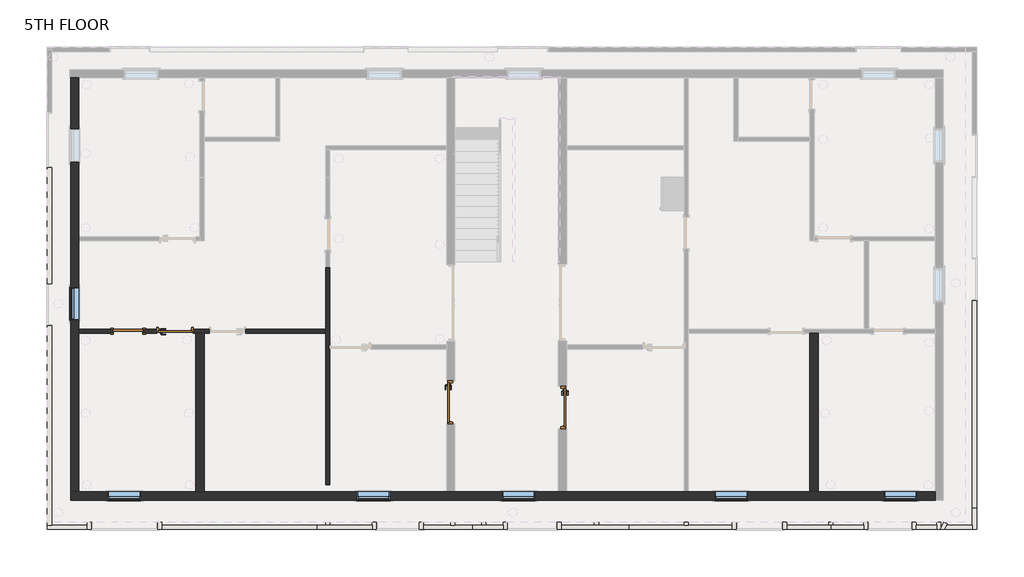
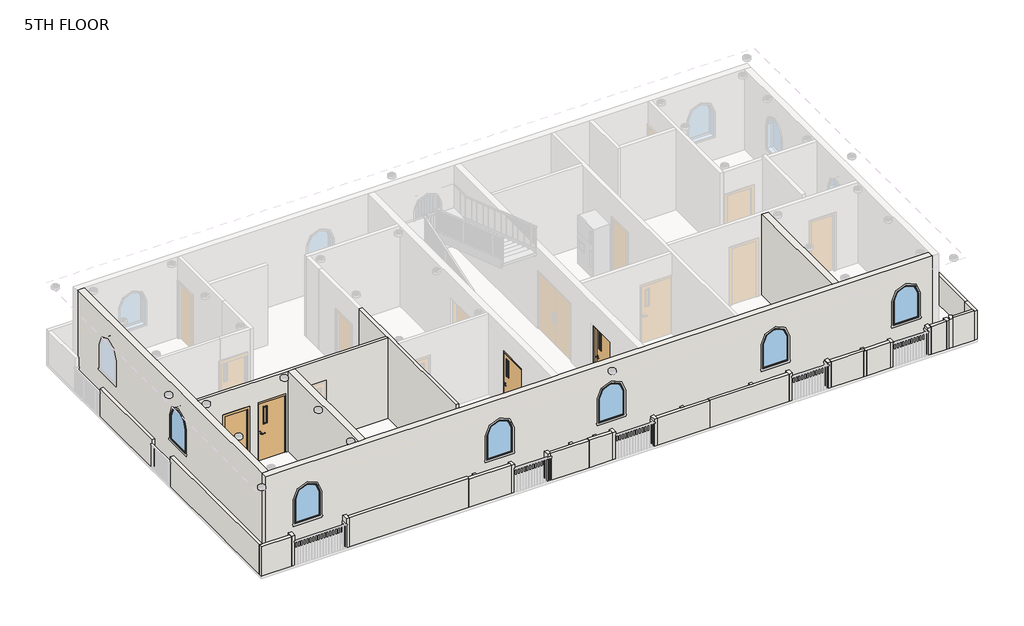
# One storey, part 1 of 7: 39 walls, 6 windows, 4 doors.
"""IFC4 building model written with IfcOpenShell, lengths in millimetres."""

from ifc_helpers import new_model, si_unit, frame, origin, place, context, project, spatial, polyline, circle_curve, outline, extrude, faceted_brep, transform, mapped, element, save
from ifc_brep_helpers import plane_surface, revolved_surface, advanced_brep
from components import door_586e558e, door_7d8f8091, door_passage_single_vision_lite_3_x7_38248cdf, door_d141acb4, window_fixed_round_top_3_x_4_dee2be1c

model = new_model("IFC4")

# Units and contexts
model_context = context("Model", 3, world=origin())
ifc_project = project(units=[si_unit("LENGTHUNIT", "METRE", prefix="MILLI")], contexts=[model_context])

# Site, building, storey
site = spatial("IfcSite", under=ifc_project)
building = spatial("IfcBuilding", under=site)
storey = spatial("IfcBuildingStorey", under=building, Name="5TH FLOOR", Elevation=16002.0)

# Doors
placement = place(None, origin())
door_shape = door_586e558e(model_context)
element("IfcDoor", 1, ObjectType="Door-Passage-Single-Vision_Lite : 3'6\"X7' 2", at=placement, inside=storey, context=model_context, shape_type="MappedRepresentation", body=[
    mapped(door_shape, transform((1116.1432011, -1461.3932193, 16002.0), x_axis=(0.0, -1.0, 0.0), y_axis=(1.0, 0.0, 0.0), z_axis=(0.0, 0.0, 1.0))),
])
door_2_shape = door_7d8f8091(model_context)
element("IfcDoor", 2, ObjectType="Door-Passage-Single-Vision_Lite : 3'7\"X7' 3", at=placement, inside=storey, context=model_context, shape_type="MappedRepresentation", body=[
    mapped(door_2_shape, transform((-1956.7487998, -1318.7421379, 16002.0), x_axis=(0.0, -1.0, 0.0), y_axis=(1.0, 0.0, 0.0), z_axis=(0.0, 0.0, 1.0))),
])
door_passage_single_vision_lite_3_x7_shape = door_passage_single_vision_lite_3_x7_38248cdf(model_context)
element("IfcDoor", 3, ObjectType="Door-Passage-Single-Vision_Lite : 3'X7'", at=placement, inside=storey, context=model_context, shape_type="MappedRepresentation", body=[
    mapped(door_passage_single_vision_lite_3_x7_shape, transform((-9570.3987992, 646.8067334, 16002.0), x_axis=(1.0, 0.0, 0.0), y_axis=(0.0, 1.0, 0.0), z_axis=(0.0, 0.0, 1.0))),
])
door_3_shape = door_d141acb4(model_context)
element("IfcDoor", 4, ObjectType="Single-Flush : 2'8\"x 7'", at=placement, inside=storey, context=model_context, shape_type="MappedRepresentation", body=[
    mapped(door_3_shape, transform((-10865.7987992, 640.4567334, 16002.0), x_axis=(1.0, 0.0, 0.0), y_axis=(0.0, 1.0, 0.0), z_axis=(0.0, 0.0, 1.0))),
])

# Walls
element("IfcWall", 5, ObjectType="Generic - 4.5\"", at=placement, inside=storey, context=model_context, shape_type="Brep", body=[
    faceted_brep([(-10459.3987992, 583.3067334, 18135.6), (-10459.3987992, 583.3067334, 16002.0), (-10078.3987992, 583.3067334, 16002.0), (-10078.3987992, 583.3067334, 18237.2), (-9062.3987992, 583.3067334, 18237.2), (-9062.3987992, 583.3067334, 16002.0), (-8998.8987992, 583.3067334, 16002.0), (-8770.2987992, 583.3067334, 16002.0), (-8630.5987992, 583.3067334, 16002.0), (-8630.5987992, 583.3067334, 18237.2), (-7614.5987992, 583.3067334, 18237.2), (-7614.5987992, 583.3067334, 16002.0), (-5417.4987995, 583.3067334, 16002.0), (-5417.4987995, 583.3067334, 19050.0), (-8770.2987992, 583.3067334, 19050.0), (-8998.8987992, 583.3067334, 19050.0), (-12224.6987925, 583.3067334, 19050.0), (-12224.6987925, 583.3067334, 16002.0), (-11272.1987992, 583.3067334, 16002.0), (-11272.1987992, 583.3067334, 18135.6), (-10078.3987992, 697.6067334, 16002.0), (-10459.3987992, 697.6067334, 16002.0), (-10459.3987992, 697.6067334, 18135.6), (-11272.1987992, 697.6067334, 18135.6), (-11272.1987992, 697.6067334, 16002.0), (-12224.6987925, 697.6067334, 16002.0), (-12224.6987925, 697.6067334, 19050.0), (-5417.4987995, 697.6067334, 19050.0), (-5417.4987995, 697.6067334, 16002.0), (-7614.5987992, 697.6067334, 16002.0), (-7614.5987992, 697.6067334, 18237.2), (-8630.5987992, 697.6067334, 18237.2), (-8630.5987992, 697.6067334, 16002.0), (-9062.3987992, 697.6067334, 16002.0), (-9062.3987992, 697.6067334, 18237.2), (-10078.3987992, 697.6067334, 18237.2)], [[[0, 1, 2, 3, 4, 5, 6, 7, 8, 9, 10, 11, 12, 13, 14, 15, 16, 17, 18, 19]], [[20, 21, 22, 23, 24, 25, 26, 27, 28, 29, 30, 31, 32, 33, 34, 35]], [[28, 12, 11, 29]], [[32, 8, 7, 6, 5, 33]], [[18, 17, 25, 24]], [[2, 1, 21, 20]], [[16, 15, 14, 13, 27, 26]], [[17, 16, 26, 25]], [[13, 12, 28, 27]], [[9, 8, 32, 31]], [[10, 9, 31, 30]], [[11, 10, 30, 29]], [[4, 34, 33, 5]], [[34, 4, 3, 35]], [[35, 3, 2, 20]], [[22, 21, 1, 0]], [[23, 22, 0, 19]], [[24, 23, 19, 18]]]),
])
element("IfcWall", 6, ObjectType="Generic - 4.5\"", at=placement, inside=storey, context=model_context, shape_type="Brep", body=[
    faceted_brep([(-5417.4987995, 2399.4067802, 16002.0), (-5417.4987995, 697.6067334, 16002.0), (-5417.4987995, 583.3067334, 16002.0), (-5417.4987995, -3594.9932193, 16002.0), (-5417.4987995, -3594.9932193, 19050.0), (-5417.4987995, 583.3067334, 19050.0), (-5417.4987995, 697.6067334, 19050.0), (-5417.4987995, 2399.4067802, 19050.0), (-5303.1987995, -3594.9932193, 19050.0), (-5303.1987995, -3594.9932193, 16002.0), (-5303.1987995, 148.1078621, 16002.0), (-5303.1987995, 148.1078621, 18237.2), (-5303.1987995, 262.4078621, 18237.2), (-5303.1987995, 262.4078621, 16002.0), (-5303.1987995, 2399.4067802, 16002.0), (-5303.1987995, 2399.4067802, 19050.0), (-5303.1987995, 262.4078621, 19050.0), (-5303.1987995, 148.1078621, 19050.0), (-5334.9487995, 262.4078621, 16002.0), (-5334.9487995, 148.1078621, 16002.0), (-5334.9487995, 262.4078621, 18237.2), (-5334.9487995, 148.1078621, 18237.2)], [[[0, 1, 2, 3, 4, 5, 6, 7]], [[8, 9, 10, 11, 12, 13, 14, 15, 16, 17]], [[3, 2, 1, 0, 14, 13, 18, 19, 10, 9]], [[4, 3, 9, 8]], [[7, 6, 5, 4, 8, 17, 16, 15]], [[0, 7, 15, 14]], [[20, 18, 13, 12]], [[19, 21, 11, 10]], [[21, 20, 12, 11]], [[18, 20, 21, 19]]]),
])
element("IfcWall", 7, ObjectType="Generic - 4.5\"", at=placement, inside=storey, context=model_context, shape_type="Brep", body=[
    faceted_brep([(-13088.8067989, -4826.8932661, 16002.0), (-11996.6067989, -4826.8932661, 16002.0), (-11996.6067989, -4826.8932661, 17114.9417562), (-13088.8067989, -4826.8932661, 17114.9417562), (-13088.8067989, -4712.5932661, 16002.0), (-13088.8067989, -4712.5932661, 17114.9417562), (-11996.6067989, -4712.5932661, 17114.9417562), (-11996.6067989, -4712.5932661, 16002.0), (-12974.5067989, -4712.5932661, 16002.0)], [[[0, 1, 2, 3]], [[4, 5, 6, 7, 8]], [[1, 0, 4, 8, 7]], [[3, 2, 6, 5]], [[2, 1, 7, 6]], [[0, 3, 5, 4]]]),
])
element("IfcWall", 8, ObjectType="Generic - 4.5\"", at=placement, inside=storey, context=model_context, shape_type="Brep", body=[
    faceted_brep([(-11996.6067989, -4623.6932193, 16002.0), (-11996.6067989, -4712.5932661, 16002.0), (-11996.6067989, -4826.8932661, 16002.0), (-11996.6067989, -4826.8932661, 17114.9417562), (-11996.6067989, -4826.8932661, 17135.9303619), (-11996.6067989, -4623.6932193, 17135.9303619), (-11882.3067989, -4623.6932193, 16002.0), (-11882.3067989, -4623.6932193, 17135.9303619), (-11882.3067989, -4826.8932661, 17135.9303619), (-11882.3067989, -4826.8932661, 16002.0)], [[[0, 1, 2, 3, 4, 5]], [[6, 7, 8, 9]], [[2, 1, 0, 6, 9]], [[5, 4, 8, 7]], [[0, 5, 7, 6]], [[4, 3, 2, 9, 8]]]),
])
element("IfcWall", 9, ObjectType="Generic - 4.5\"", at=placement, inside=storey, context=model_context, shape_type="Brep", body=[
    faceted_brep([(11660.3143245, -4826.8932661, 16002.0), (12426.0012043, -4826.8932661, 16002.0), (12426.0012043, -4826.8932661, 17093.8617784), (12426.0012043, -4826.8932661, 17105.1196614), (11660.3143245, -4826.8932661, 17105.1196614), (11660.3143245, -4826.8932661, 17091.5342527), (11716.0621594, -4712.5932661, 16002.0), (11716.0621594, -4712.5932661, 17105.1196614), (12426.0012043, -4712.5932661, 17105.1196614), (12426.0012043, -4712.5932661, 16002.0)], [[[0, 1, 2, 3, 4, 5]], [[6, 7, 8, 9]], [[1, 0, 6, 9]], [[4, 3, 8, 7]], [[3, 2, 1, 9, 8]], [[0, 5, 4, 7, 6]]]),
])
element("IfcWall", 10, ObjectType="Generic - 4.5\"", at=placement, inside=storey, context=model_context, shape_type="Brep", body=[
    faceted_brep([(11632.2512075, -4623.6932193, 16002.0), (11533.1439227, -4826.8932661, 16002.0), (11533.1439227, -4826.8932661, 17091.5342527), (11632.2512075, -4623.6932193, 17091.5342527), (11734.983367, -4673.7990414, 16002.0), (11734.983367, -4673.7990414, 17091.5342527), (11660.3143245, -4826.8932661, 17091.5342527), (11660.3143245, -4826.8932661, 16002.0), (11716.0621594, -4712.5932661, 16002.0)], [[[0, 1, 2, 3]], [[4, 5, 6, 7, 8]], [[1, 0, 4, 8, 7]], [[3, 2, 6, 5]], [[0, 3, 5, 4]], [[2, 1, 7, 6]]]),
])
element("IfcWall", 11, ObjectType="Generic - 4.5\"", at=placement, inside=storey, context=model_context, shape_type="Brep", body=[
    faceted_brep([(12426.0012043, -4236.3432661, 16002.0), (12426.0012043, -4712.5932661, 16002.0), (12426.0012043, -4826.8932661, 16002.0), (12426.0012043, -4826.8932661, 17093.8617784), (12426.0012043, -4236.3432661, 17093.8617784), (12426.0012043, -4236.3432661, 17088.6712164), (12540.3012043, -4236.3432661, 16002.0), (12540.3012043, -4236.3432661, 17088.6712164), (12540.3012043, -4236.3432661, 17093.8617784), (12540.3012043, -4826.8932661, 17093.8617784), (12540.3012043, -4826.8932661, 16002.0)], [[[0, 1, 2, 3, 4, 5]], [[6, 7, 8, 9, 10]], [[2, 1, 0, 6, 10]], [[4, 3, 9, 8]], [[0, 5, 4, 8, 7, 6]], [[3, 2, 10, 9]]]),
])
element("IfcWall", 12, ObjectType="Generic - 4.5\"", at=placement, inside=storey, context=model_context, shape_type="SweptSolid", body=[
    extrude(outline(polyline([(-5417.4987995, -4712.5932661), (-5417.4987995, -4623.6932193), (-5303.1987995, -4623.6932193), (-5303.1987995, -4712.5932661), (-5417.4987995, -4712.5932661)])), frame((0.0, 0.0, 16002.0), z_axis=(0.0, 0.0, 1.0), x_axis=(1.0, 0.0, 0.0)), (0.0, 0.0, 1.0), 1063.0786215),
])
element("IfcWall", 13, ObjectType="Generic - 4.5\"", at=placement, inside=storey, context=model_context, shape_type="Brep", body=[
    faceted_brep([(-5663.8033402, -4826.8932661, 16002.0), (-4134.7987995, -4826.8932661, 16002.0), (-4134.7987995, -4826.8932661, 17061.1218247), (-4134.7987995, -4826.8932661, 17069.2575049), (-5663.8033402, -4826.8932661, 17069.2575049), (-5663.8033402, -4712.5932661, 16002.0), (-5663.8033402, -4712.5932661, 17069.2575049), (-4134.7987995, -4712.5932661, 17069.2575049), (-4134.7987995, -4712.5932661, 16002.0), (-5303.1987995, -4712.5932661, 16002.0), (-5417.4987995, -4712.5932661, 16002.0)], [[[0, 1, 2, 3, 4]], [[5, 6, 7, 8, 9, 10]], [[1, 0, 5, 10, 9, 8]], [[4, 3, 7, 6]], [[0, 4, 6, 5]], [[3, 2, 1, 8, 7]]]),
])
element("IfcWall", 14, ObjectType="Generic - 4.5\"", at=placement, inside=storey, context=model_context, shape_type="Brep", body=[
    faceted_brep([(-2725.0987995, -4826.8932661, 16002.0), (-1354.4417672, -4826.8932661, 16002.0), (-1354.4417672, -4826.8932661, 17018.0), (-2725.0987995, -4826.8932661, 17018.0), (-2725.0987995, -4712.5932661, 16002.0), (-2725.0987995, -4712.5932661, 17018.0), (-1354.4417672, -4712.5932661, 17018.0), (-1354.4417672, -4712.5932661, 16002.0), (-1848.7987998, -4712.5932661, 16002.0), (-1963.0987998, -4712.5932661, 16002.0)], [[[0, 1, 2, 3]], [[4, 5, 6, 7, 8, 9]], [[1, 0, 4, 9, 8, 7]], [[2, 1, 7, 6]], [[3, 2, 6, 5]], [[0, 3, 5, 4]]]),
])
element("IfcWall", 15, ObjectType="Generic - 4.5\"", at=placement, inside=storey, context=model_context, shape_type="SweptSolid", body=[
    extrude(outline(polyline([(-1963.0987998, -4712.5932661), (-1963.0987998, -4623.6932193), (-1848.7987998, -4623.6932193), (-1848.7987998, -4712.5932661), (-1963.0987998, -4712.5932661)])), frame((0.0, 0.0, 16002.0), z_axis=(0.0, 0.0, 1.0), x_axis=(1.0, 0.0, 0.0)), (0.0, 0.0, 1.0), 1029.3234006),
])
element("IfcWall", 16, ObjectType="Generic - 4.5\"", at=placement, inside=storey, context=model_context, shape_type="SweptSolid", body=[
    extrude(outline(polyline([(-1112.1987998, -4712.5932661), (-1112.1987998, -4623.6932193), (-997.8987998, -4623.6932193), (-997.8987998, -4712.5932661), (-1112.1987998, -4712.5932661)])), frame((0.0, 0.0, 16002.0), z_axis=(0.0, 0.0, 1.0), x_axis=(1.0, 0.0, 0.0)), (0.0, 0.0, 1.0), 1016.0),
])
element("IfcWall", 17, ObjectType="Generic - 4.5\"", at=placement, inside=storey, context=model_context, shape_type="SweptSolid", body=[
    extrude(outline(polyline([(1999.3012002, -4712.5932661), (1999.3012002, -4623.6932193), (2113.6012002, -4623.6932193), (2113.6012002, -4712.5932661), (1999.3012002, -4712.5932661)])), frame((0.0, 0.0, 16002.0), z_axis=(0.0, 0.0, 1.0), x_axis=(1.0, 0.0, 0.0)), (0.0, 0.0, 1.0), 1013.2250283),
])
element("IfcWall", 18, ObjectType="Generic - 4.5\"", at=placement, inside=storey, context=model_context, shape_type="SweptSolid", body=[
    extrude(outline(polyline([(4475.8012082, -4712.5932661), (4475.8012082, -4623.6932193), (4590.1012082, -4623.6932193), (4590.1012082, -4712.5932661), (4475.8012082, -4712.5932661)])), frame((0.0, 0.0, 16002.0), z_axis=(0.0, 0.0, 1.0), x_axis=(1.0, 0.0, 0.0)), (0.0, 0.0, 1.0), 1027.4591445),
])
element("IfcWall", 19, ObjectType="Generic - 4.5\"", at=placement, inside=storey, context=model_context, shape_type="Brep", body=[
    faceted_brep([(2962.6087812, -4826.8932661, 16002.0), (5802.9512082, -4826.8932661, 16002.0), (5802.9512082, -4826.8932661, 17029.4591445), (2962.6087812, -4826.8932661, 17029.4591445), (2962.6087812, -4826.8932661, 17015.2250283), (2962.6087812, -4712.5932661, 16002.0), (2962.6087812, -4712.5932661, 17015.2250283), (2962.6087812, -4712.5932661, 17029.4591445), (4475.8012082, -4712.5932661, 17029.4591445), (4590.1012082, -4712.5932661, 17029.4591445), (5802.9512082, -4712.5932661, 17029.4591445), (5802.9512082, -4712.5932661, 16002.0), (4590.1012082, -4712.5932661, 16002.0), (4475.8012082, -4712.5932661, 16002.0)], [[[0, 1, 2, 3, 4]], [[5, 6, 7, 8, 9, 10, 11, 12, 13]], [[1, 0, 5, 13, 12, 11]], [[3, 2, 10, 9, 8, 7]], [[0, 4, 3, 7, 6, 5]], [[2, 1, 11, 10]]]),
])
element("IfcWall", 20, ObjectType="Generic - 4.5\"", at=placement, inside=storey, context=model_context, shape_type="Brep", body=[
    faceted_brep([(5802.9512082, -4623.6932193, 16002.0), (5802.9512082, -4712.5932661, 16002.0), (5802.9512082, -4826.8932661, 16002.0), (5802.9512082, -4826.8932661, 17029.4591445), (5802.9512082, -4826.8932661, 17034.3822201), (5802.9512082, -4623.6932193, 17034.3822201), (5917.2512082, -4623.6932193, 16002.0), (5917.2512082, -4623.6932193, 17034.3822201), (5917.2512082, -4826.8932661, 17034.3822201), (5917.2512082, -4826.8932661, 16002.0)], [[[0, 1, 2, 3, 4, 5]], [[6, 7, 8, 9]], [[2, 1, 0, 6, 9]], [[5, 4, 8, 7]], [[0, 5, 7, 6]], [[4, 3, 2, 9, 8]]]),
])
element("IfcWall", 21, ObjectType="Generic - 4.5\"", at=placement, inside=storey, context=model_context, shape_type="Brep", body=[
    faceted_brep([(7190.3011643, -4623.6932193, 16002.0), (7190.3011643, -4826.8932661, 16002.0), (7190.3011643, -4826.8932661, 16974.8158009), (7190.3011643, -4623.6932193, 16974.8158009), (7304.6011643, -4623.6932193, 16002.0), (7304.6011643, -4623.6932193, 16974.8158009), (7304.6011643, -4712.5932661, 16974.8158009), (7304.6011643, -4826.8932661, 16974.8158009), (7304.6011643, -4826.8932661, 16002.0), (7304.6011643, -4712.5932661, 16002.0)], [[[0, 1, 2, 3]], [[4, 5, 6, 7, 8, 9]], [[1, 0, 4, 9, 8]], [[3, 2, 7, 6, 5]], [[0, 3, 5, 4]], [[2, 1, 8, 7]]]),
])
element("IfcWall", 22, ObjectType="Generic - 4.5\"", at=placement, inside=storey, context=model_context, shape_type="Brep", body=[
    faceted_brep([(7304.6011643, -4826.8932661, 16002.0), (8463.6012082, -4826.8932661, 16002.0), (8463.6012082, -4826.8932661, 16958.4159658), (8520.7512082, -4826.8932661, 16958.4159658), (8520.7512082, -4826.8932661, 16971.680309), (8520.7512082, -4826.8932661, 16974.9581334), (7304.6011643, -4826.8932661, 16974.9581334), (7304.6011643, -4712.5932661, 16002.0), (7304.6011643, -4712.5932661, 16974.9581334), (8520.7512082, -4712.5932661, 16974.9581334), (8520.7512082, -4712.5932661, 16971.680309), (8520.7512082, -4712.5932661, 16958.4159658), (8463.6012082, -4712.5932661, 16958.4159658), (8463.6012082, -4712.5932661, 16002.0)], [[[0, 1, 2, 3, 4, 5, 6]], [[7, 8, 9, 10, 11, 12, 13]], [[1, 0, 7, 13]], [[6, 5, 9, 8]], [[0, 6, 8, 7]], [[5, 4, 3, 11, 10, 9]], [[11, 3, 2, 12]], [[2, 1, 13, 12]]]),
])
element("IfcWall", 23, ObjectType="Generic - 4.5\"", at=placement, inside=storey, context=model_context, shape_type="Brep", body=[
    faceted_brep([(8463.6012082, -4623.6932193, 16002.0), (8463.6012082, -4712.5932661, 16002.0), (8463.6012082, -4826.8932661, 16002.0), (8463.6012082, -4826.8932661, 16958.4159658), (8463.6012082, -4712.5932661, 16958.4159658), (8463.6012082, -4623.6932193, 16958.4159658), (8577.9012082, -4623.6932193, 16002.0), (8577.9012082, -4623.6932193, 16958.4159658), (8577.9012082, -4712.5932661, 16958.4159658), (8577.9012082, -4826.8932661, 16958.4159658), (8577.9012082, -4826.8932661, 16002.0), (8577.9012082, -4712.5932661, 16002.0), (8520.7512082, -4826.8932661, 16958.4159658)], [[[0, 1, 2, 3, 4, 5]], [[6, 7, 8, 9, 10, 11]], [[2, 1, 0, 6, 11, 10]], [[5, 4, 3, 12, 9, 8, 7]], [[0, 5, 7, 6]], [[3, 2, 10, 9, 12]]]),
])
element("IfcWall", 24, ObjectType="Generic - 4.5\"", at=placement, inside=storey, context=model_context, shape_type="Brep", body=[
    faceted_brep([(8577.9012082, -4826.8932661, 16002.0), (9422.4512082, -4826.8932661, 16002.0), (9422.4512082, -4826.8932661, 16954.2060641), (9422.4512082, -4826.8932661, 16971.680309), (8520.7512082, -4826.8932661, 16971.680309), (8520.7512082, -4826.8932661, 16958.4159658), (8577.9012082, -4826.8932661, 16958.4159658), (8577.9012082, -4712.5932661, 16002.0), (8577.9012082, -4712.5932661, 16958.4159658), (8520.7512082, -4712.5932661, 16958.4159658), (8520.7512082, -4712.5932661, 16971.680309), (9422.4512082, -4712.5932661, 16971.680309), (9422.4512082, -4712.5932661, 16002.0)], [[[0, 1, 2, 3, 4, 5, 6]], [[7, 8, 9, 10, 11, 12]], [[1, 0, 7, 12]], [[4, 3, 11, 10]], [[3, 2, 1, 12, 11]], [[5, 4, 10, 9]], [[5, 9, 8, 6]], [[0, 6, 8, 7]]]),
])
element("IfcWall", 25, ObjectType="Generic - 4.5\"", at=placement, inside=storey, context=model_context, shape_type="Brep", body=[
    faceted_brep([(9422.4512082, -4623.6932193, 16002.0), (9422.4512082, -4712.5932661, 16002.0), (9422.4512082, -4826.8932661, 16002.0), (9422.4512082, -4826.8932661, 16954.2060641), (9422.4512082, -4623.6932193, 16954.2060641), (9536.7512082, -4623.6932193, 16002.0), (9536.7512082, -4623.6932193, 16954.2060641), (9536.7512082, -4826.8932661, 16954.2060641), (9536.7512082, -4826.8932661, 16002.0)], [[[0, 1, 2, 3, 4]], [[5, 6, 7, 8]], [[2, 1, 0, 5, 8]], [[4, 3, 7, 6]], [[0, 4, 6, 5]], [[3, 2, 8, 7]]]),
])
element("IfcWall", 26, ObjectType="Generic - 4.5\"", at=placement, inside=storey, context=model_context, shape_type="Brep", body=[
    faceted_brep([(10764.1617205, -4623.6932193, 16002.0), (10764.1617205, -4826.8932661, 16002.0), (10764.1617205, -4826.8932661, 17028.3072304), (10764.1617205, -4623.6932193, 17028.3072304), (10878.4617205, -4623.6932193, 16002.0), (10878.4617205, -4623.6932193, 17028.3072304), (10878.4617205, -4826.8932661, 17028.3072304), (10878.4617205, -4826.8932661, 16002.0), (10878.4617205, -4712.5932661, 16002.0)], [[[0, 1, 2, 3]], [[4, 5, 6, 7, 8]], [[1, 0, 4, 8, 7]], [[3, 2, 6, 5]], [[0, 3, 5, 4]], [[2, 1, 7, 6]]]),
])
element("IfcWall", 27, ObjectType="Generic - 4.5\"", at=placement, inside=storey, context=model_context, shape_type="Brep", body=[
    faceted_brep([(10878.4617205, -4826.8932661, 16002.0), (11437.2617205, -4826.8932661, 16002.0), (11437.2617205, -4826.8932661, 17050.6912221), (10878.4617205, -4826.8932661, 17050.6912221), (10878.4617205, -4826.8932661, 17028.3072304), (10878.4617205, -4712.5932661, 16002.0), (10878.4617205, -4712.5932661, 17050.6912221), (11437.2617205, -4712.5932661, 17050.6912221), (11437.2617205, -4712.5932661, 16002.0)], [[[0, 1, 2, 3, 4]], [[5, 6, 7, 8]], [[1, 0, 5, 8]], [[3, 2, 7, 6]], [[0, 4, 3, 6, 5]], [[2, 1, 8, 7]]]),
])
element("IfcWall", 28, ObjectType="Generic - 4.5\"", at=placement, inside=storey, context=model_context, shape_type="Brep", body=[
    faceted_brep([(11437.2617205, -4623.6932193, 16002.0), (11437.2617205, -4712.5932661, 16002.0), (11437.2617205, -4826.8932661, 16002.0), (11437.2617205, -4826.8932661, 17050.6912221), (11437.2617205, -4712.5932661, 17050.6912221), (11437.2617205, -4623.6932193, 17050.6912221), (11551.5617205, -4623.6932193, 16002.0), (11551.5617205, -4623.6932193, 17050.6912221), (11551.5617205, -4826.8932661, 17050.6912221), (11551.5617205, -4826.8932661, 16002.0)], [[[0, 1, 2, 3, 4, 5]], [[6, 7, 8, 9]], [[2, 1, 0, 6, 9]], [[5, 4, 3, 8, 7]], [[0, 5, 7, 6]], [[3, 2, 9, 8]]]),
])
element("IfcWall", 29, ObjectType="Generic - 4.5\"", at=placement, inside=storey, context=model_context, shape_type="Brep", body=[
    faceted_brep([(-4134.7987995, -4623.6932193, 16002.0), (-4134.7987995, -4712.5932661, 16002.0), (-4134.7987995, -4826.8932661, 16002.0), (-4134.7987995, -4826.8932661, 17061.1218247), (-4134.7987995, -4623.6932193, 17061.1218247), (-4020.4987995, -4623.6932193, 16002.0), (-4020.4987995, -4623.6932193, 17061.1218247), (-4020.4987995, -4826.8932661, 17061.1218247), (-4020.4987995, -4826.8932661, 16002.0)], [[[0, 1, 2, 3, 4]], [[5, 6, 7, 8]], [[2, 1, 0, 5, 8]], [[4, 3, 7, 6]], [[0, 4, 6, 5]], [[3, 2, 8, 7]]]),
])
element("IfcWall", 30, ObjectType="Generic - 4.5\"", at=placement, inside=storey, context=model_context, shape_type="Brep", body=[
    faceted_brep([(-2839.3987995, -4623.6932193, 16002.0), (-2839.3987995, -4826.8932661, 16002.0), (-2839.3987995, -4826.8932661, 17018.7549618), (-2839.3987995, -4623.6932193, 17018.7549618), (-2725.0987995, -4623.6932193, 16002.0), (-2725.0987995, -4623.6932193, 17018.7549618), (-2725.0987995, -4826.8932661, 17018.7549618), (-2725.0987995, -4826.8932661, 17018.0), (-2725.0987995, -4826.8932661, 16002.0), (-2725.0987995, -4712.5932661, 16002.0)], [[[0, 1, 2, 3]], [[4, 5, 6, 7, 8, 9]], [[1, 0, 4, 9, 8]], [[3, 2, 6, 5]], [[0, 3, 5, 4]], [[2, 1, 8, 7, 6]]]),
])
element("IfcWall", 31, ObjectType="Generic - 4.5\"", at=placement, inside=storey, context=model_context, shape_type="Brep", body=[
    faceted_brep([(-1354.4417672, -4826.8932661, 16002.0), (-520.5065315, -4826.8932661, 16002.0), (-520.5065315, -4826.8932661, 17025.8796817), (-520.5065315, -4826.8932661, 17033.140074), (-1354.4417672, -4826.8932661, 17033.140074), (-1354.4417672, -4826.8932661, 17018.0), (-1354.4417672, -4712.5932661, 16002.0), (-1354.4417672, -4712.5932661, 17018.0), (-1354.4417672, -4712.5932661, 17033.140074), (-520.5065315, -4712.5932661, 17033.140074), (-520.5065315, -4712.5932661, 16002.0), (-997.8987998, -4712.5932661, 16002.0), (-1112.1987998, -4712.5932661, 16002.0)], [[[0, 1, 2, 3, 4, 5]], [[6, 7, 8, 9, 10, 11, 12]], [[1, 0, 6, 12, 11, 10]], [[4, 3, 9, 8]], [[0, 5, 4, 8, 7, 6]], [[3, 2, 1, 10, 9]]]),
])
element("IfcWall", 32, ObjectType="Generic - 4.5\"", at=placement, inside=storey, context=model_context, shape_type="Brep", body=[
    faceted_brep([(-520.5065315, -4623.6932193, 16002.0), (-520.5065315, -4712.5932661, 16002.0), (-520.5065315, -4826.8932661, 16002.0), (-520.5065315, -4826.8932661, 17025.8796817), (-520.5065315, -4623.6932193, 17025.8796817), (-406.2065315, -4623.6932193, 16002.0), (-406.2065315, -4623.6932193, 17025.8796817), (-406.2065315, -4826.8932661, 17025.8796817), (-406.2065315, -4826.8932661, 16002.0)], [[[0, 1, 2, 3, 4]], [[5, 6, 7, 8]], [[2, 1, 0, 5, 8]], [[4, 3, 7, 6]], [[0, 4, 6, 5]], [[3, 2, 8, 7]]]),
])
element("IfcWall", 33, ObjectType="Generic - 4.5\"", at=placement, inside=storey, context=model_context, shape_type="Brep", body=[
    faceted_brep([(970.0932011, -4623.6932193, 16002.0), (970.0932011, -4826.8932661, 16002.0), (970.0932011, -4826.8932661, 17015.2250283), (970.0932011, -4623.6932193, 17015.2250283), (1084.3932011, -4623.6932193, 16002.0), (1084.3932011, -4623.6932193, 17015.2250283), (1084.3932011, -4712.5932661, 17015.2250283), (1084.3932011, -4826.8932661, 17015.2250283), (1084.3932011, -4826.8932661, 16002.0), (1084.3932011, -4712.5932661, 16002.0)], [[[0, 1, 2, 3]], [[4, 5, 6, 7, 8, 9]], [[1, 0, 4, 9, 8]], [[3, 2, 7, 6, 5]], [[0, 3, 5, 4]], [[2, 1, 8, 7]]]),
])
element("IfcWall", 34, ObjectType="Generic - 4.5\"", at=placement, inside=storey, context=model_context, shape_type="Brep", body=[
    faceted_brep([(1084.3932011, -4826.8932661, 16002.0), (2962.6087812, -4826.8932661, 16002.0), (2962.6087812, -4826.8932661, 17015.2250283), (1084.3932011, -4826.8932661, 17015.2250283), (1084.3932011, -4712.5932661, 16002.0), (1084.3932011, -4712.5932661, 17015.2250283), (1999.3012002, -4712.5932661, 17015.2250283), (2113.6012002, -4712.5932661, 17015.2250283), (2962.6087812, -4712.5932661, 17015.2250283), (2962.6087812, -4712.5932661, 16002.0), (2113.6012002, -4712.5932661, 16002.0), (1999.3012002, -4712.5932661, 16002.0)], [[[0, 1, 2, 3]], [[4, 5, 6, 7, 8, 9, 10, 11]], [[1, 0, 4, 11, 10, 9]], [[2, 1, 9, 8]], [[3, 2, 8, 7, 6, 5]], [[0, 3, 5, 4]]]),
])
element("IfcWall", 35, ObjectType="Generic - 4.5\"", at=placement, inside=storey, context=model_context, shape_type="Brep", body=[
    faceted_brep([(-10045.9470335, -4623.6932193, 16002.0), (-10045.9470335, -4826.8932661, 16002.0), (-10045.9470335, -4826.8932661, 17109.704535), (-10045.9470335, -4623.6932193, 17109.704535), (-9931.6470335, -4623.6932193, 16002.0), (-9931.6470335, -4623.6932193, 17109.704535), (-9931.6470335, -4712.5932661, 17109.704535), (-9931.6470335, -4826.8932661, 17109.704535), (-9931.6470335, -4826.8932661, 16002.0), (-9931.6470335, -4712.5932661, 16002.0)], [[[0, 1, 2, 3]], [[4, 5, 6, 7, 8, 9]], [[1, 0, 4, 9, 8]], [[3, 2, 7, 6, 5]], [[0, 3, 5, 4]], [[2, 1, 8, 7]]]),
])
element("IfcWall", 36, ObjectType="Generic - 4.5\"", at=placement, inside=storey, context=model_context, shape_type="Brep", body=[
    faceted_brep([(-9931.6470335, -4826.8932661, 16002.0), (-5663.8033402, -4826.8932661, 16002.0), (-5663.8033402, -4826.8932661, 17069.2575049), (-5663.8033402, -4826.8932661, 17109.704535), (-9931.6470335, -4826.8932661, 17109.704535), (-9931.6470335, -4712.5932661, 16002.0), (-9931.6470335, -4712.5932661, 17109.704535), (-5663.8033402, -4712.5932661, 17109.704535), (-5663.8033402, -4712.5932661, 17069.2575049), (-5663.8033402, -4712.5932661, 16002.0)], [[[0, 1, 2, 3, 4]], [[5, 6, 7, 8, 9]], [[1, 0, 5, 9]], [[3, 2, 1, 9, 8, 7]], [[4, 3, 7, 6]], [[0, 4, 6, 5]]]),
])
element("IfcWall", 37, ObjectType="Generic - 4.5\"", at=placement, inside=storey, context=model_context, shape_type="Brep", body=[
    faceted_brep([(-13088.8067989, 792.8567339, 16002.0), (-13088.8067989, -4712.5932661, 16002.0), (-13088.8067989, -4712.5932661, 17114.9417562), (-13088.8067989, -4712.5932661, 17116.167936), (-13088.8067989, 792.8567339, 17116.167936), (-12974.5067989, 792.8567339, 16002.0), (-12974.5067989, 792.8567339, 17116.167936), (-12974.5067989, -4712.5932661, 17116.167936), (-12974.5067989, -4712.5932661, 16002.0)], [[[0, 1, 2, 3, 4]], [[5, 6, 7, 8]], [[1, 0, 5, 8]], [[4, 3, 7, 6]], [[0, 4, 6, 5]], [[3, 2, 1, 8, 7]]]),
])
element("IfcWall", 38, ObjectType="Generic - 4.5\"", at=placement, inside=storey, context=model_context, shape_type="SweptSolid", body=[
    extrude(outline(polyline([(-12976.0338648, 5154.3604213), (-12976.0338648, 1953.9604213), (-13090.3338648, 1953.9604213), (-13090.3338648, 5154.3604213), (-12976.0338648, 5154.3604213)])), frame((0.0, 0.0, 16002.0), z_axis=(0.0, 0.0, 1.0), x_axis=(1.0, 0.0, 0.0)), (0.0, 0.0, 1.0), 1047.4413329),
])
element("IfcWall", 39, ObjectType="Generic - 4.5\"", at=placement, inside=storey, context=model_context, shape_type="SweptSolid", body=[
    extrude(outline(polyline([(12426.0012043, -4236.3432661), (12426.0012043, 1478.6567334), (12540.3012043, 1478.6567334), (12540.3012043, -4236.3432661), (12426.0012043, -4236.3432661)])), frame((0.0, 0.0, 16002.0), z_axis=(0.0, 0.0, 1.0), x_axis=(1.0, 0.0, 0.0)), (0.0, 0.0, 1.0), 1086.6712164),
])
element("IfcWall", 40, ObjectType="Generic - 9\"", at=placement, inside=storey, context=model_context, shape_type="AdvancedBrep", body=[
    advanced_brep(
    [(11397.3012075, -3785.4932193, 16002.0), (8171.5012079, -3785.4932193, 16002.0), (7942.9012079, -3785.4932193, 16002.0), (4590.1012082, -3785.4932193, 16002.0), (4475.8012082, -3785.4932193, 16002.0), (1236.7932011, -3785.4932193, 16002.0), (1008.1932011, -3785.4932193, 16002.0), (-1848.7987998, -3785.4932193, 16002.0), (-2077.3987998, -3785.4932193, 16002.0), (-8770.2987992, -3785.4932193, 16002.0), (-8998.8987992, -3785.4932193, 16002.0), (-12224.6987925, -3785.4932193, 16002.0), (-12453.2987925, -3785.4932193, 16002.0), (-12453.2987925, -3785.4932193, 19050.0), (-12224.6987925, -3785.4932193, 19050.0), (-8998.8987992, -3785.4932193, 19050.0), (-8770.2987992, -3785.4932193, 19050.0), (-2077.3987998, -3785.4932193, 19050.0), (-1848.7987998, -3785.4932193, 19050.0), (1008.1932011, -3785.4932193, 19050.0), (1236.7932011, -3785.4932193, 19050.0), (4475.8012082, -3785.4932193, 19050.0), (4590.1012082, -3785.4932193, 19050.0), (7942.9012079, -3785.4932193, 19050.0), (8171.5012079, -3785.4932193, 19050.0), (11397.3012075, -3785.4932193, 19050.0), (-10510.1987925, -3785.4932193, 16916.4), (-10510.1987925, -3785.4932193, 17830.8), (-11424.5987925, -3785.4932193, 17830.8), (-11424.5987925, -3785.4932193, 16916.4), (-3639.4987998, -3785.4932193, 16916.4), (-3639.4987998, -3785.4932193, 17830.8), (-4553.8987998, -3785.4932193, 17830.8), (-4553.8987998, -3785.4932193, 16916.4), (360.4932011, -3785.4932193, 16916.4), (360.4932011, -3785.4932193, 17830.8), (-553.9067989, -3785.4932193, 17830.8), (-553.9067989, -3785.4932193, 16916.4), (6228.4012079, -3785.4932193, 16916.4), (6228.4012079, -3785.4932193, 17830.8), (5314.0012079, -3785.4932193, 17830.8), (5314.0012079, -3785.4932193, 16916.4), (10902.0012075, -3785.4932193, 16916.4), (10902.0012075, -3785.4932193, 17830.8), (9987.6012075, -3785.4932193, 17830.8), (9987.6012075, -3785.4932193, 16916.4), (11397.3012075, -4014.0932193, 16002.0), (11397.3012075, -4014.0932193, 19050.0), (-12453.2987925, -4014.0932193, 19050.0), (-12453.2987925, -4014.0932193, 16002.0), (-10510.1987925, -4014.0932193, 16916.4), (-11424.5987925, -4014.0932193, 16916.4), (-11424.5987925, -4014.0932193, 17830.8), (-10510.1987925, -4014.0932193, 17830.8), (-3639.4987998, -4014.0932193, 16916.4), (-4553.8987998, -4014.0932193, 16916.4), (-4553.8987998, -4014.0932193, 17830.8), (-3639.4987998, -4014.0932193, 17830.8), (360.4932011, -4014.0932193, 16916.4), (-553.9067989, -4014.0932193, 16916.4), (-553.9067989, -4014.0932193, 17830.8), (360.4932011, -4014.0932193, 17830.8), (6228.4012079, -4014.0932193, 16916.4), (5314.0012079, -4014.0932193, 16916.4), (5314.0012079, -4014.0932193, 17830.8), (6228.4012079, -4014.0932193, 17830.8), (10902.0012075, -4014.0932193, 16916.4), (9987.6012075, -4014.0932193, 16916.4), (9987.6012075, -4014.0932193, 17830.8), (10902.0012075, -4014.0932193, 17830.8)],
    [
        (0, 1),
        (1, 2),
        (2, 3),
        (3, 4),
        (4, 5),
        (5, 6),
        (6, 7),
        (7, 8),
        (8, 9),
        (9, 10),
        (10, 11),
        (11, 12),
        (12, 13),
        (13, 14),
        (14, 15),
        (15, 16),
        (16, 17),
        (17, 18),
        (18, 19),
        (19, 20),
        (20, 21),
        (21, 22),
        (22, 23),
        (23, 24),
        (24, 25),
        (25, 0),
        (26, 27),
        (27, 28, circle_curve(frame((-10967.3987925, -3785.4932193, 17830.8), z_axis=(0.0, -1.0, 0.0), x_axis=(-1.0, 0.0, 0.0)), 457.2)),
        (28, 29),
        (29, 26),
        (30, 31),
        (31, 32, circle_curve(frame((-4096.6987998, -3785.4932193, 17830.8), z_axis=(0.0, -1.0, 0.0), x_axis=(-1.0, 0.0, 0.0)), 457.2)),
        (32, 33),
        (33, 30),
        (34, 35),
        (35, 36, circle_curve(frame((-96.7067989, -3785.4932193, 17830.8), z_axis=(0.0, -1.0, 0.0), x_axis=(-1.0, 0.0, 0.0)), 457.2)),
        (36, 37),
        (37, 34),
        (38, 39),
        (39, 40, circle_curve(frame((5771.2012079, -3785.4932193, 17830.8), z_axis=(0.0, -1.0, 0.0), x_axis=(-1.0, 0.0, 0.0)), 457.2)),
        (40, 41),
        (41, 38),
        (42, 43),
        (43, 44, circle_curve(frame((10444.8012075, -3785.4932193, 17830.8), z_axis=(0.0, -1.0, 0.0), x_axis=(-1.0, 0.0, 0.0)), 457.2)),
        (44, 45),
        (45, 42),
        (46, 47),
        (47, 48),
        (48, 49),
        (49, 46),
        (50, 51),
        (51, 52),
        (52, 53, circle_curve(frame((-10967.3987925, -4014.0932193, 17830.8), z_axis=(0.0, 1.0, 0.0), x_axis=(-1.0, 0.0, 0.0)), 457.2)),
        (53, 50),
        (54, 55),
        (55, 56),
        (56, 57, circle_curve(frame((-4096.6987998, -4014.0932193, 17830.8), z_axis=(0.0, 1.0, 0.0), x_axis=(-1.0, 0.0, 0.0)), 457.2)),
        (57, 54),
        (58, 59),
        (59, 60),
        (60, 61, circle_curve(frame((-96.7067989, -4014.0932193, 17830.8), z_axis=(0.0, 1.0, 0.0), x_axis=(-1.0, 0.0, 0.0)), 457.2)),
        (61, 58),
        (62, 63),
        (63, 64),
        (64, 65, circle_curve(frame((5771.2012079, -4014.0932193, 17830.8), z_axis=(0.0, 1.0, 0.0), x_axis=(-1.0, 0.0, 0.0)), 457.2)),
        (65, 62),
        (66, 67),
        (67, 68),
        (68, 69, circle_curve(frame((10444.8012075, -4014.0932193, 17830.8), z_axis=(0.0, 1.0, 0.0), x_axis=(-1.0, 0.0, 0.0)), 457.2)),
        (69, 66),
        (0, 46),
        (49, 12),
        (13, 48),
        (47, 25),
        (50, 26),
        (29, 51),
        (28, 52),
        (27, 53),
        (54, 30),
        (33, 55),
        (32, 56),
        (31, 57),
        (58, 34),
        (37, 59),
        (36, 60),
        (35, 61),
        (62, 38),
        (41, 63),
        (40, 64),
        (39, 65),
        (66, 42),
        (45, 67),
        (44, 68),
        (43, 69),
    ],
    [
        plane_surface(frame((11386.6090247, -3785.4932193, 16002.0), z_axis=(0.0, 1.0, 0.0), x_axis=(-1.0, 0.0, 0.0))),
        plane_surface(frame((11386.6090247, -4014.0932193, 16002.0), z_axis=(0.0, -1.0, 0.0), x_axis=(1.0, 0.0, 0.0))),
        plane_surface(frame((11511.6012075, -3785.4932193, 16002.0), z_axis=(0.0, 0.0, -1.0), x_axis=(0.0, -1.0, 0.0))),
        plane_surface(frame((-12338.9987925, -3785.4932193, 19050.0), z_axis=(0.0, 0.0, 1.0), x_axis=(0.0, -1.0, 0.0))),
        plane_surface(frame((11397.3012075, 7629.6366753, 16002.0), z_axis=(1.0, 0.0, 0.0), x_axis=(0.0, -1.0, 0.0))),
        plane_surface(frame((-12453.2987925, -3782.6829884, 16002.0), z_axis=(-1.0, 0.0, 0.0), x_axis=(0.0, -1.0, 0.0))),
        plane_surface(frame((-10510.1987925, -4014.0932193, 16916.4), z_axis=(0.0, 0.0, 1.0), x_axis=(0.0, 1.0, 0.0))),
        plane_surface(frame((-11424.5987925, -4014.0932193, 16916.4), z_axis=(1.0, 0.0, 0.0), x_axis=(0.0, 1.0, 0.0))),
        revolved_surface(polyline([(-11424.5987925, -3785.4932193, 17830.8), (-11424.5987925, -4014.0932193, 17830.8)]), (-10967.3987925, -3785.4932193, 17830.8), (0.0, 1.0, 0.0)),
        plane_surface(frame((-10510.1987925, -4014.0932193, 17830.8), z_axis=(-1.0, 0.0, 0.0), x_axis=(0.0, 1.0, 0.0))),
        plane_surface(frame((-3639.4987998, -4014.0932193, 16916.4), z_axis=(0.0, 0.0, 1.0), x_axis=(0.0, 1.0, 0.0))),
        plane_surface(frame((-4553.8987998, -4014.0932193, 16916.4), z_axis=(1.0, 0.0, 0.0), x_axis=(0.0, 1.0, 0.0))),
        revolved_surface(polyline([(-4553.8987998, -3785.4932193, 17830.8), (-4553.8987998, -4014.0932193, 17830.8)]), (-4096.6987998, -3785.4932193, 17830.8), (0.0, 1.0, 0.0)),
        plane_surface(frame((-3639.4987998, -4014.0932193, 17830.8), z_axis=(-1.0, 0.0, 0.0), x_axis=(0.0, 1.0, 0.0))),
        plane_surface(frame((360.4932011, -4014.0932193, 16916.4), z_axis=(0.0, 0.0, 1.0), x_axis=(0.0, 1.0, 0.0))),
        plane_surface(frame((-553.9067989, -4014.0932193, 16916.4), z_axis=(1.0, 0.0, 0.0), x_axis=(0.0, 1.0, 0.0))),
        revolved_surface(polyline([(-553.9067989, -3785.4932193, 17830.8), (-553.9067989, -4014.0932193, 17830.8)]), (-96.7067989, -3785.4932193, 17830.8), (0.0, 1.0, 0.0)),
        plane_surface(frame((360.4932011, -4014.0932193, 17830.8), z_axis=(-1.0, 0.0, 0.0), x_axis=(0.0, 1.0, 0.0))),
        plane_surface(frame((6228.4012079, -4014.0932193, 16916.4), z_axis=(0.0, 0.0, 1.0), x_axis=(0.0, 1.0, 0.0))),
        plane_surface(frame((5314.0012079, -4014.0932193, 16916.4), z_axis=(1.0, 0.0, 0.0), x_axis=(0.0, 1.0, 0.0))),
        revolved_surface(polyline([(5314.0012079, -3785.4932193, 17830.8), (5314.0012079, -4014.0932193, 17830.8)]), (5771.2012079, -3785.4932193, 17830.8), (0.0, 1.0, 0.0)),
        plane_surface(frame((6228.4012079, -4014.0932193, 17830.8), z_axis=(-1.0, 0.0, 0.0), x_axis=(0.0, 1.0, 0.0))),
        plane_surface(frame((10902.0012075, -4014.0932193, 16916.4), z_axis=(0.0, 0.0, 1.0), x_axis=(0.0, 1.0, 0.0))),
        plane_surface(frame((9987.6012075, -4014.0932193, 16916.4), z_axis=(1.0, 0.0, 0.0), x_axis=(0.0, 1.0, 0.0))),
        revolved_surface(polyline([(9987.6012075, -3785.4932193, 17830.8), (9987.6012075, -4014.0932193, 17830.8)]), (10444.8012075, -3785.4932193, 17830.8), (0.0, 1.0, 0.0)),
        plane_surface(frame((10902.0012075, -4014.0932193, 17830.8), z_axis=(-1.0, 0.0, 0.0), x_axis=(0.0, 1.0, 0.0))),
    ],
    [
        (0, [[1, 2, 3, 4, 5, 6, 7, 8, 9, 10, 11, 12, 13, 14, 15, 16, 17, 18, 19, 20, 21, 22, 23, 24, 25, 26], [27, 28, 29, 30], [31, 32, 33, 34], [35, 36, 37, 38], [39, 40, 41, 42], [43, 44, 45, 46]]),
        (1, [[47, 48, 49, 50], [51, 52, 53, 54], [55, 56, 57, 58], [59, 60, 61, 62], [63, 64, 65, 66], [67, 68, 69, 70]]),
        (2, [[-12, -11, -10, -9, -8, -7, -6, -5, -4, -3, -2, -1, 71, -50, 72]]),
        (3, [[-25, -24, -23, -22, -21, -20, -19, -18, -17, -16, -15, -14, 73, -48, 74]]),
        (4, [[-26, -74, -47, -71]]),
        (5, [[-13, -72, -49, -73]]),
        (6, [[-51, 75, -30, 76]]),
        (7, [[-52, -76, -29, 77]]),
        (8, [[-53, -77, -28, 78]]),
        (9, [[-54, -78, -27, -75]]),
        (10, [[-55, 79, -34, 80]]),
        (11, [[-56, -80, -33, 81]]),
        (12, [[-57, -81, -32, 82]]),
        (13, [[-58, -82, -31, -79]]),
        (14, [[-59, 83, -38, 84]]),
        (15, [[-60, -84, -37, 85]]),
        (16, [[-61, -85, -36, 86]]),
        (17, [[-62, -86, -35, -83]]),
        (18, [[-63, 87, -42, 88]]),
        (19, [[-64, -88, -41, 89]]),
        (20, [[-65, -89, -40, 90]]),
        (21, [[-66, -90, -39, -87]]),
        (22, [[-67, 91, -46, 92]]),
        (23, [[-68, -92, -45, 93]]),
        (24, [[-69, -93, -44, 94]]),
        (25, [[-70, -94, -43, -91]]),
    ],
),
])
element("IfcWall", 41, ObjectType="Generic - 9\"", at=placement, inside=storey, context=model_context, shape_type="AdvancedBrep", body=[
    advanced_brep(
    [(-12224.6987925, -3785.4932193, 16002.0), (-12224.6987925, 583.3067334, 16002.0), (-12224.6987925, 697.6067334, 16002.0), (-12224.6987925, 3136.0067332, 16002.0), (-12224.6987925, 3250.3067332, 16002.0), (-12224.6987925, 7631.8067329, 16002.0), (-12224.6987925, 7631.8067329, 19050.0), (-12224.6987925, 3250.3067332, 19050.0), (-12224.6987925, 3136.0067332, 19050.0), (-12224.6987925, 697.6067334, 19050.0), (-12224.6987925, 583.3067334, 19050.0), (-12224.6987925, -3785.4932193, 19050.0), (-12224.6987925, 5307.7067329, 16916.4), (-12224.6987925, 5307.7067329, 17830.8), (-12224.6987925, 6222.1067329, 17830.8), (-12224.6987925, 6222.1067329, 16916.4), (-12224.6987925, 945.2567334, 16916.4), (-12224.6987925, 945.2567334, 17830.8), (-12224.6987925, 1859.6567334, 17830.8), (-12224.6987925, 1859.6567334, 16916.4), (-12453.2987925, -3785.4932193, 16002.0), (-12453.2987925, -3785.4932193, 19050.0), (-12453.2987925, 7631.8067329, 19050.0), (-12453.2987925, 7631.8067329, 16002.0), (-12453.2987925, 5307.7067329, 16916.4), (-12453.2987925, 6222.1067329, 16916.4), (-12453.2987925, 6222.1067329, 17830.8), (-12453.2987925, 5307.7067329, 17830.8), (-12453.2987925, 945.2567334, 16916.4), (-12453.2987925, 1859.6567334, 16916.4), (-12453.2987925, 1859.6567334, 17830.8), (-12453.2987925, 945.2567334, 17830.8)],
    [
        (0, 1),
        (1, 2),
        (2, 3),
        (3, 4),
        (4, 5),
        (5, 6),
        (6, 7),
        (7, 8),
        (8, 9),
        (9, 10),
        (10, 11),
        (11, 0),
        (12, 13),
        (13, 14, circle_curve(frame((-12224.6987925, 5764.9067329, 17830.8), z_axis=(-1.0, 0.0, 0.0), x_axis=(0.0, 1.0, 0.0)), 457.2)),
        (14, 15),
        (15, 12),
        (16, 17),
        (17, 18, circle_curve(frame((-12224.6987925, 1402.4567334, 17830.8), z_axis=(-1.0, 0.0, 0.0), x_axis=(0.0, 1.0, 0.0)), 457.2)),
        (18, 19),
        (19, 16),
        (20, 21),
        (21, 22),
        (22, 23),
        (23, 20),
        (24, 25),
        (25, 26),
        (26, 27, circle_curve(frame((-12453.2987925, 5764.9067329, 17830.8), z_axis=(1.0, 0.0, 0.0), x_axis=(0.0, 1.0, 0.0)), 457.2)),
        (27, 24),
        (28, 29),
        (29, 30),
        (30, 31, circle_curve(frame((-12453.2987925, 1402.4567334, 17830.8), z_axis=(1.0, 0.0, 0.0), x_axis=(0.0, 1.0, 0.0)), 457.2)),
        (31, 28),
        (0, 20),
        (23, 5),
        (6, 22),
        (21, 11),
        (24, 12),
        (15, 25),
        (14, 26),
        (13, 27),
        (28, 16),
        (19, 29),
        (18, 30),
        (17, 31),
    ],
    [
        plane_surface(frame((-12224.6987925, -3782.6829884, 16002.0), z_axis=(1.0, 0.0, 0.0), x_axis=(0.0, 1.0, 0.0))),
        plane_surface(frame((-12453.2987925, -3782.6829884, 16002.0), z_axis=(-1.0, 0.0, 0.0), x_axis=(0.0, -1.0, 0.0))),
        plane_surface(frame((-12224.6987925, -3899.7932193, 16002.0), z_axis=(0.0, 0.0, -1.0), x_axis=(-1.0, 0.0, 0.0))),
        plane_surface(frame((-12224.6987925, 7746.1067329, 19050.0), z_axis=(0.0, 0.0, 1.0), x_axis=(-1.0, 0.0, 0.0))),
        plane_surface(frame((11386.6090247, -3785.4932193, 16002.0), z_axis=(0.0, -1.0, 0.0), x_axis=(-1.0, 0.0, 0.0))),
        plane_surface(frame((-12479.2067989, 7631.8067329, 16002.0), z_axis=(0.0, 1.0, 0.0), x_axis=(1.0, 0.0, 0.0))),
        plane_surface(frame((-12453.2987925, 5307.7067329, 16916.4), z_axis=(0.0, 0.0, 1.0), x_axis=(1.0, 0.0, 0.0))),
        plane_surface(frame((-12453.2987925, 6222.1067329, 16916.4), z_axis=(0.0, -1.0, 0.0), x_axis=(1.0, 0.0, 0.0))),
        revolved_surface(polyline([(-12224.6987925, 6222.1067329, 17830.8), (-12453.2987925, 6222.1067329, 17830.8)]), (-12224.6987925, 5764.9067329, 17830.8), (1.0, 0.0, 0.0)),
        plane_surface(frame((-12453.2987925, 5307.7067329, 17830.8), z_axis=(0.0, 1.0, 0.0), x_axis=(1.0, 0.0, 0.0))),
        plane_surface(frame((-12453.2987925, 945.2567334, 16916.4), z_axis=(0.0, 0.0, 1.0), x_axis=(1.0, 0.0, 0.0))),
        plane_surface(frame((-12453.2987925, 1859.6567334, 16916.4), z_axis=(0.0, -1.0, 0.0), x_axis=(1.0, 0.0, 0.0))),
        revolved_surface(polyline([(-12224.6987925, 1859.6567334000001, 17830.8), (-12453.2987925, 1859.6567334000001, 17830.8)]), (-12224.6987925, 1402.4567334, 17830.8), (1.0, 0.0, 0.0)),
        plane_surface(frame((-12453.2987925, 945.2567334, 17830.8), z_axis=(0.0, 1.0, 0.0), x_axis=(1.0, 0.0, 0.0))),
    ],
    [
        (0, [[1, 2, 3, 4, 5, 6, 7, 8, 9, 10, 11, 12], [13, 14, 15, 16], [17, 18, 19, 20]]),
        (1, [[21, 22, 23, 24], [25, 26, 27, 28], [29, 30, 31, 32]]),
        (2, [[-5, -4, -3, -2, -1, 33, -24, 34]]),
        (3, [[-11, -10, -9, -8, -7, 35, -22, 36]]),
        (4, [[-12, -36, -21, -33]]),
        (5, [[-6, -34, -23, -35]]),
        (6, [[-25, 37, -16, 38]]),
        (7, [[-26, -38, -15, 39]]),
        (8, [[-27, -39, -14, 40]]),
        (9, [[-28, -40, -13, -37]]),
        (10, [[-29, 41, -20, 42]]),
        (11, [[-30, -42, -19, 43]]),
        (12, [[-31, -43, -18, 44]]),
        (13, [[-32, -44, -17, -41]]),
    ],
),
])
element("IfcWall", 42, ObjectType="Generic - 9\"", at=placement, inside=storey, context=model_context, shape_type="SweptSolid", body=[
    extrude(outline(polyline([(-8998.8987992, -3785.4932193), (-8998.8987992, 583.3067334), (-8770.2987992, 583.3067334), (-8770.2987992, -3785.4932193), (-8998.8987992, -3785.4932193)])), frame((0.0, 0.0, 16002.0), z_axis=(0.0, 0.0, 1.0), x_axis=(1.0, 0.0, 0.0)), (0.0, 0.0, 1.0), 3048.0),
])
element("IfcWall", 43, ObjectType="Generic - 9\"", at=placement, inside=storey, context=model_context, shape_type="SweptSolid", body=[
    extrude(outline(polyline([(7942.9012079, -3785.4932193), (7942.9012079, 583.3067334), (8171.5012079, 583.3067334), (8171.5012079, -3785.4932193), (7942.9012079, -3785.4932193)])), frame((0.0, 0.0, 16002.0), z_axis=(0.0, 0.0, 1.0), x_axis=(1.0, 0.0, 0.0)), (0.0, 0.0, 1.0), 3048.0),
])

# Windows
window_fixed_round_top_3_x_4_shape = window_fixed_round_top_3_x_4_dee2be1c(model_context)
element("IfcWindow", 44, ObjectType="Window-Fixed-Round-Top : 3' x 4'", at=placement, inside=storey, context=model_context, shape_type="MappedRepresentation", body=[
    mapped(window_fixed_round_top_3_x_4_shape, transform((-10967.3987925, -3899.7932193, 16002.0), x_axis=(-1.0, 0.0, 0.0), y_axis=(0.0, -1.0, 0.0), z_axis=(0.0, 0.0, 1.0))),
])
element("IfcWindow", 45, ObjectType="Window-Fixed-Round-Top : 3' x 4'", at=placement, inside=storey, context=model_context, shape_type="MappedRepresentation", body=[
    mapped(window_fixed_round_top_3_x_4_shape, transform((-4096.6987998, -3899.7932193, 16002.0), x_axis=(-1.0, 0.0, 0.0), y_axis=(0.0, -1.0, 0.0), z_axis=(0.0, 0.0, 1.0))),
])
element("IfcWindow", 46, ObjectType="Window-Fixed-Round-Top : 3' x 4'", at=placement, inside=storey, context=model_context, shape_type="MappedRepresentation", body=[
    mapped(window_fixed_round_top_3_x_4_shape, transform((-96.7067989, -3899.7932193, 16002.0), x_axis=(-1.0, 0.0, 0.0), y_axis=(0.0, -1.0, 0.0), z_axis=(0.0, 0.0, 1.0))),
])
element("IfcWindow", 47, ObjectType="Window-Fixed-Round-Top : 3' x 4'", at=placement, inside=storey, context=model_context, shape_type="MappedRepresentation", body=[
    mapped(window_fixed_round_top_3_x_4_shape, transform((5771.2012079, -3899.7932193, 16002.0), x_axis=(-1.0, 0.0, 0.0), y_axis=(0.0, -1.0, 0.0), z_axis=(0.0, 0.0, 1.0))),
])
element("IfcWindow", 48, ObjectType="Window-Fixed-Round-Top : 3' x 4'", at=placement, inside=storey, context=model_context, shape_type="MappedRepresentation", body=[
    mapped(window_fixed_round_top_3_x_4_shape, transform((10444.8012075, -3899.7932193, 16002.0), x_axis=(-1.0, 0.0, 0.0), y_axis=(0.0, -1.0, 0.0), z_axis=(0.0, 0.0, 1.0))),
])
element("IfcWindow", 49, ObjectType="Window-Fixed-Round-Top : 3' x 4'", at=placement, inside=storey, context=model_context, shape_type="MappedRepresentation", body=[
    mapped(window_fixed_round_top_3_x_4_shape, transform((-12338.9987925, 1402.4567334, 16002.0), x_axis=(0.0, 1.0, 0.0), y_axis=(-1.0, 0.0, 0.0), z_axis=(0.0, 0.0, 1.0))),
])

save(model, "model.ifc")

# Revit data of these elements
# Type "Door-Passage-Single-Vision_Lite : 3'6\"X7' 2"
#   Type Mark = "14"
#   Assembly Code = "B2030100"
#   Analytic Construction = "Wooden"
#   Thickness = 0' - 1 3/4"
#   Thermal Resistance (R) = 2.5876 (h·ft²·°F)/BTU
#   Swing Angle [instance default] = 90.00°
#   Strike Height = 3' - 4"
#   Rough Width [instance default] = 3' - 10"
#   Rough Height [instance default] = 7' - 4"
#   MFOpeningHeight [instance default] = 0' - 4"
#   MFOpeningWidth [instance default] = 0' - 4"
#   Inset Calculate [instance default] = 0' - 4"
#   Masonry Inset [instance default] = 0' - 1"
#   Height = 7' - 0"
#   Width = 3' - 6"
#   Heat Transfer Coefficient (U) = 0.3865 BTU/(h·ft²·°F)
#   Masonry Frame Depth = 0' - 5 3/4"
#   Masonry Frame [instance default] = yes
#   Function = 1
#   Dry Wall Frame [instance default] = no
#   Panel Material = Wood - Birch
#   Glazing = Glass
#   Glass Stop Material = Metal - Paint Finish - Grey
#   Frame Material = Metal - Paint Finish - Grey
#   Door Handle Material = Aluminum
#   Visual Light Transmittance = 0
#   Solar Heat Gain Coefficient = 0
#   Wall Closure = (empty or 0)
# Type "Door-Passage-Single-Vision_Lite : 3'7\"X7' 3"
#   Type Mark = "15"
#   Assembly Code = "B2030100"
#   Analytic Construction = "Wooden"
#   Thickness = 0' - 1 3/4"
#   Thermal Resistance (R) = 2.5876 (h·ft²·°F)/BTU
#   Swing Angle [instance default] = 90.00°
#   Strike Height = 3' - 4"
#   Rough Width [instance default] = 3' - 11"
#   Rough Height [instance default] = 7' - 4"
#   MFOpeningHeight [instance default] = 0' - 4"
#   MFOpeningWidth [instance default] = 0' - 4"
#   Inset Calculate [instance default] = 0' - 4"
#   Masonry Inset [instance default] = 0' - 1"
#   Height = 7' - 0"
#   Width = 3' - 7"
#   Heat Transfer Coefficient (U) = 0.3865 BTU/(h·ft²·°F)
#   Masonry Frame Depth = 0' - 5 3/4"
#   Masonry Frame [instance default] = yes
#   Function = 1
#   Dry Wall Frame [instance default] = no
#   Panel Material = Wood - Birch
#   Glazing = Glass
#   Glass Stop Material = Metal - Paint Finish - Grey
#   Frame Material = Metal - Paint Finish - Grey
#   Door Handle Material = Aluminum
#   Visual Light Transmittance = 0
#   Solar Heat Gain Coefficient = 0
#   Wall Closure = (empty or 0)
# Type "Door-Passage-Single-Vision_Lite : 3'X7'"
#   Type Mark = "9"
#   Assembly Code = "B2030100"
#   Analytic Construction = "Wooden"
#   Thickness = 0' - 1 3/4"
#   Thermal Resistance (R) = 2.5876 (h·ft²·°F)/BTU
#   Swing Angle [instance default] = 90.00°
#   Strike Height = 3' - 4"
#   Rough Width [instance default] = 3' - 4"
#   Rough Height [instance default] = 7' - 4"
#   MFOpeningHeight [instance default] = 0' - 4"
#   MFOpeningWidth [instance default] = 0' - 4"
#   Inset Calculate [instance default] = 0' - 4"
#   Masonry Inset [instance default] = 0' - 1"
#   Height = 7' - 0"
#   Width = 3' - 0"
#   Heat Transfer Coefficient (U) = 0.3865 BTU/(h·ft²·°F)
#   Masonry Frame Depth = 0' - 5 3/4"
#   Masonry Frame [instance default] = yes
#   Function = 1
#   Dry Wall Frame [instance default] = no
#   Panel Material = Wood - Birch
#   Glazing = Glass
#   Glass Stop Material = Metal - Paint Finish - Grey
#   Frame Material = Metal - Paint Finish - Grey
#   Door Handle Material = Aluminum
#   Visual Light Transmittance = 0
#   Solar Heat Gain Coefficient = 0
#   Wall Closure = (empty or 0)
# Type "Single-Flush : 2'8\"x 7'"
#   Type Mark = "11"
#   Construction Type Id = "MDOOR"
#   Assembly Code = "C1020"
#   Analytic Construction = "Metal"
#   Thickness = 0' - 2"
#   Heat Transfer Coefficient (U) = 0.651978 BTU/(h·ft²·°F)
#   Height = 7' - 0"
#   Trim Projection Ext = 0' - 1"
#   Trim Projection Int = 0' - 1"
#   Trim Width = 0' - 3"
#   Width = 2' - 8"
#   Define Thermal Properties by = 1
#   Door Material = Door - Panel
#   Frame Material = Door - Frame
#   Visual Light Transmittance = 0
#   Solar Heat Gain Coefficient = 0
#   Function = (empty or 0)
#   Wall Closure = (empty or 0)
# Type "Generic - 4.5\""
#   Assembly Code = "B2010"
#   Layers, outside or top first: 0' - 4 1/2" no material (function 1)
# Type "Generic - 9\""
#   Assembly Code = "B2010"
#   Layers, outside or top first: 0' - 9" "Concrete Masonry Units" (function 1)
# Type "Window-Fixed-Round-Top : 3' x 4'"
#   Type Mark = "21"
#   Fire Rating = "0.5h"
#   Assembly Code = "B2020100"
#   Analytic Construction = "Double glazing - domestic"
#   Window Inset [instance default] = 0' - 0"
#   Wall Thickness [instance default] = 0' - 6"
#   Visual Light Transmittance = 0.81
#   Thermal Resistance (R) = 1.8146 (h·ft²·°F)/BTU
#   Solar Heat Gain Coefficient = 0.76
#   Rough Width = 3' - 0 1/2"
#   Rough Height = 4' - 6 1/2"
#   Interior Wall Closure [instance default] = 0' - 2 1/4"
#   Height = 4' - 6"
#   Heat Transfer Coefficient (U) = 0.5511 BTU/(h·ft²·°F)
#   Frame Extension [instance default] = 0' - 0 1/4"
#   Exterior Wall Closure [instance default] = 0' - 1 1/4"
#   Extension Jamb [instance default] = 0' - 2 1/4"
#   Default Sill Height = 3' - 0"
#   Width = 3' - 0"
#   Interior Trim Visibility [instance default] = yes
#   Exterior Trim Visibility [instance default] = yes
#   Extension Jamb Visibility [instance default] = yes
#   Interior Trim Material = Wood - Stained
#   Interior Trim = Trim-Window-Interior-Flat-Arch-Top-Tree_Centered : Picture Frame
#   Interior Frame Material = Wood - Stained
#   Glass Panel Material = Glass
#   Exterior Trim Material = Clad - White
#   Exterior Trim = Trim-Window-Exterior-Flat-Arch-Top-Tree_Centered : with Sill
#   Exterior Frame Material = Clad - White
#   Wall Closure = (empty or 0)
# Element 1 (IfcDoor, "Door-Passage-Single-Vision_Lite : 3'6\"X7' 2")
#   Swing Angle = 90.00°
#   Rough Width = 3' - 10"
#   Rough Height = 7' - 4"
#   Masonry Inset = 0' - 1"
#   MFOpeningWidth = 0' - 4"
#   MFOpeningHeight = 0' - 4"
#   Inset Calculate = 0' - 4"
#   Masonry Frame = yes
#   Dry Wall Frame = no
#   Phase Created = New Construction
#   Materials on its faces: "Metal - Paint Finish - Grey", "Aluminum", "Wood - Birch", "Glass"
# Element 2 (IfcDoor, "Door-Passage-Single-Vision_Lite : 3'7\"X7' 3")
#   Swing Angle = 90.00°
#   Rough Width = 3' - 11"
#   Rough Height = 7' - 4"
#   Masonry Inset = 0' - 1"
#   MFOpeningWidth = 0' - 4"
#   MFOpeningHeight = 0' - 4"
#   Inset Calculate = 0' - 4"
#   Masonry Frame = yes
#   Dry Wall Frame = no
#   Phase Created = New Construction
#   Materials on its faces: "Metal - Paint Finish - Grey", "Aluminum", "Wood - Birch", "Glass"
# Element 3 (IfcDoor, "Door-Passage-Single-Vision_Lite : 3'X7'")
#   Swing Angle = 90.00°
#   Rough Width = 3' - 4"
#   Rough Height = 7' - 4"
#   Masonry Inset = 0' - 1"
#   MFOpeningWidth = 0' - 4"
#   MFOpeningHeight = 0' - 4"
#   Inset Calculate = 0' - 4"
#   Masonry Frame = yes
#   Dry Wall Frame = no
#   Phase Created = New Construction
#   Materials on its faces: "Metal - Paint Finish - Grey", "Aluminum", "Wood - Birch", "Glass"
# Element 4 (IfcDoor, "Single-Flush : 2'8\"x 7'")
